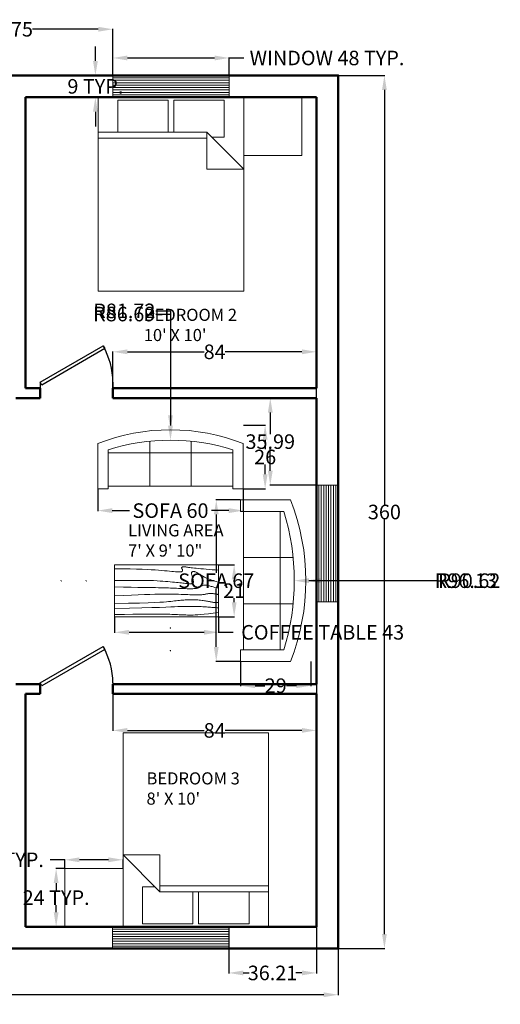
# Model space of a CAD drawing. Units: inches. Extents: x -8 to 445, y -363 to 43.
# Tile 3 of 3: x 246 to 445, y -363 to 43. Entities that reach past the tile are written whole.
import ezdxf

# ---------------------------------------------------------------- set-up
doc = ezdxf.new("R2010")
doc.units = ezdxf.units.IN
doc.header["$MEASUREMENT"] = 0
for name, color, linetype, lineweight in [('A-ANNO-DIMS', 2, 'Continuous', 18), ('A-AREA-IDEN', 7, 'Continuous', 18), ('A-FURN', 8, 'Continuous', 18), ('A-WALL', 7, 'Continuous', 50), ('DOORS', 43, 'Continuous', 25), ('WINDOWS', 140, 'Continuous', 18)]:
    doc.layers.add(name, color=color, linetype=linetype, lineweight=lineweight)
doc.styles.get("Standard").update_dxf_attribs({"font": 'arial.ttf'})
doc.dimstyles.get("Standard").update_dxf_attribs({"dimtxt": 6, "dimasz": 6, "dimexe": 0.18, "dimexo": 0.0625, "dimgap": 0.09, "dimtad": 0, "dimtih": 1, "dimtoh": 1, "dimdec": 0, "dimzin": 0, "dimdsep": 46, "dimlunit": 4, "dimtxsty": 'Standard', "dimcen": 0.09, "dimadec": 0, "dimazin": 0, "dimtfac": 1, "dimtdec": 0, "dimtofl": 0, "dimtmove": 0, "dimatfit": 3, "dimfxl": 1, "dimtolj": 1, "dimtzin": 0, "dimarcsym": 0})

# ---------------------------------------------------------------- blocks, each defined once
blk = doc.blocks.new('*U2')
for p, q in [((0, 0), (0, -6)), ((40, 0), (40, -6))]:
    blk.add_line(p, q)
blk.add_lwpolyline([(0, 0), (34.64, 20), (35.52, 18.48), (0.87, -1.52)], close=True)
blk.add_arc((0, 0), 40, 0, 30)
blk = doc.blocks.new('Sofa - Roundback 7 ft.')
for p, q in [((-12.00002, -32.4421), (-12.00003, -6.5971)), ((11.99997, -32.4421), (11.99998, -6.5971)), ((-36.000027, -34), (-36.000027, -11.4696)), ((-35.999844, -13.3819), (35.9998, -13.3819)), ((35.99998, -34), (35.99998, -11.4696)), ((-36.000027, -32.4421), (35.99998, -32.4421))]:
    blk.add_line(p, q)
for points in [[(-36.000027, -34), (-42.000027, -34), (-42.000027, -8)], [(41.99998, -8), (41.99998, -34), (35.99998, -34)]]:
    blk.add_lwpolyline(points)
for centre, radius, start, end in [((0, -114.25), 114.25, 68.43141, 111.5686), ((-0.00001, -127.1968), 121.1968, 72.72033, 107.2797)]:
    blk.add_arc(centre, radius, start, end)
blk = doc.blocks.new('Table - Rectangular Woodgrain 60 x 30 in.')
for p, q in [((0, 0), (0, -30)), ((60, 0), (0, 0)), ((60, -30), (60, 0)), ((0, -30), (60, -30))]:
    blk.add_line(p, q)
for points in [[(0, -2.4), (4.8155, -2.418), (9.0302, -2.4688), (12.709, -2.5477), (15.9167, -2.65), (18.7181, -2.7711), (21.1781, -2.9063), (23.3616, -3.0508), (25.3333, -3.2), (27.1477, -3.3495), (28.8172, -3.4958), (30.3437, -3.636), (31.7291, -3.7667), (32.9756, -3.8849), (34.0849, -3.9875), (35.059, -4.0714), (35.9, -4.1334), (36.6114, -4.1711), (37.2041, -4.1854), (37.6906, -4.1779), (38.0833, -4.15), (38.3948, -4.1034), (38.6375, -4.0396), (38.8239, -3.9602), (38.9666, -3.8667), (39.0764, -3.7608), (39.1573, -3.6448), (39.2116, -3.521), (39.2416, -3.3917), (39.2498, -3.2593), (39.2385, -3.1261), (39.21, -2.9944), (39.1666, -2.8667), (39.111, -2.7447), (39.0468, -2.6281), (38.978, -2.5163), (38.9083, -2.4083), (38.8418, -2.3035), (38.7823, -2.201), (38.7337, -2.1001), (38.7, -2), (38.6844, -1.9003), (38.6875, -1.8021), (38.7094, -1.707), (38.75, -1.6167), (38.8094, -1.5326), (38.8875, -1.4563), (38.9844, -1.3893), (39.1, -1.3333), (39.2351, -1.2896), (39.3937, -1.2583), (39.5804, -1.2396), (39.8, -1.2333), (40.057, -1.2396), (40.3562, -1.2583), (40.7023, -1.2896), (41.1, -1.3333), (41.5547, -1.3895), (42.0755, -1.4573), (42.6721, -1.5361), (43.3542, -1.625), (44.1316, -1.7233), (45.014, -1.8302), (46.0114, -1.9449), (47.1333, -2.0667), (48.3862, -2.1947), (49.7625, -2.3281), (51.2513, -2.4663), (52.8416, -2.6083), (54.5226, -2.7535), (56.2833, -2.9011), (58.1127, -3.0501), (60, -3.2)], [(0, -9.2), (6.5759, -9.0858), (11.9385, -9.0365), (16.2527, -9.0418), (19.6833, -9.0917), (22.3952, -9.1759), (24.5531, -9.2844), (26.322, -9.4069), (27.8666, -9.5333), (29.3241, -9.6553), (30.7203, -9.7719), (32.0532, -9.8837), (33.3208, -9.9917), (34.5213, -10.0965), (35.6526, -10.199), (36.7128, -10.2999), (37.7, -10.4), (38.6129, -10.4996), (39.4531, -10.5969), (40.223, -10.6895), (40.925, -10.775), (41.5613, -10.8512), (42.1344, -10.9156), (42.6465, -10.966), (43.1, -11), (43.4976, -11.0158), (43.8437, -11.0136), (44.143, -10.9942), (44.4, -10.9583), (44.6195, -10.9069), (44.8062, -10.8406), (44.9648, -10.7603), (45.1, -10.6667), (45.2155, -10.5598), (45.3114, -10.4365), (45.3871, -10.2929), (45.4416, -10.125), (45.4743, -9.929), (45.4844, -9.7011), (45.4709, -9.4371), (45.4333, -9.1333), (45.3716, -8.7883), (45.2896, -8.4104), (45.1919, -8.0107), (45.0833, -7.6), (44.9685, -7.1893), (44.8521, -6.7896), (44.7388, -6.4117), (44.6333, -6.0667), (44.54, -5.7628), (44.4614, -5.4979), (44.4001, -5.2675), (44.3583, -5.0667), (44.3384, -4.8909), (44.3427, -4.7354), (44.3736, -4.5956), (44.4333, -4.4667), (44.5236, -4.3453), (44.6427, -4.2333), (44.7884, -4.1339), (44.9583, -4.05), (45.1501, -3.9849), (45.3614, -3.9417), (45.59, -3.9234), (45.8333, -3.9333), (46.0915, -3.9749), (46.3734, -4.0531), (46.6906, -4.1736), (47.0542, -4.3417), (47.4756, -4.5629), (47.9661, -4.8427), (48.5372, -5.1866), (49.2, -5.6), (49.9676, -6.0844), (50.8594, -6.625), (51.8965, -7.2031), (53.1, -7.8), (54.491, -8.3969), (56.0906, -8.975), (57.9199, -9.5156), (60, -10)], [(0, -12.8), (5.1847, -12.9322), (9.6213, -13.0323), (13.3963, -13.1059), (16.5958, -13.1583), (19.3063, -13.1952), (21.614, -13.2219), (23.6054, -13.2439), (25.3666, -13.2667), (26.9728, -13.2947), (28.4531, -13.3281), (29.8256, -13.3663), (31.1083, -13.4083), (32.3191, -13.4535), (33.476, -13.501), (34.597, -13.5501), (35.7, -13.6), (36.7984, -13.6497), (37.8875, -13.6979), (38.9578, -13.743), (40, -13.7833), (41.0047, -13.8174), (41.9625, -13.8438), (42.864, -13.8607), (43.7, -13.8667), (44.4631, -13.8604), (45.1552, -13.8417), (45.7801, -13.8104), (46.3416, -13.7667), (46.8439, -13.7104), (47.2906, -13.6417), (47.6858, -13.5604), (48.0333, -13.4667), (48.3375, -13.3608), (48.6042, -13.2448), (48.8396, -13.121), (49.05, -12.9917), (49.2417, -12.8593), (49.4208, -12.7261), (49.5937, -12.5944), (49.7667, -12.4667), (49.9452, -12.3451), (50.1323, -12.2313), (50.3303, -12.1268), (50.5416, -12.0333), (50.7686, -11.9524), (51.0135, -11.8854), (51.2788, -11.8341), (51.5666, -11.8), (51.8785, -11.7843), (52.2116, -11.7865), (52.562, -11.8059), (52.926, -11.8417), (53.2998, -11.8931), (53.6795, -11.9594), (54.0614, -12.0397), (54.4416, -12.1333), (54.8223, -12.2401), (55.2293, -12.3625), (55.6942, -12.5037), (56.2489, -12.6667), (56.9251, -12.8547), (57.7545, -13.0708), (58.7689, -13.3182), (60, -13.6)], [(0, -18), (5.124, -17.7273), (9.6609, -17.5057), (13.6705, -17.3303), (17.2125, -17.1958), (20.3467, -17.0973), (23.1328, -17.0297), (25.6307, -16.9878), (27.9, -16.9667), (29.9928, -16.9617), (31.9302, -16.9703), (33.7254, -16.9907), (35.3917, -17.0208), (36.9423, -17.0588), (38.3906, -17.1026), (39.7499, -17.1503), (41.0333, -17.2), (42.2519, -17.2496), (43.4073, -17.2969), (44.4986, -17.3395), (45.525, -17.375), (46.4858, -17.4012), (47.3802, -17.4156), (48.2074, -17.416), (48.9667, -17.4), (49.6583, -17.3662), (50.2872, -17.3167), (50.8595, -17.2547), (51.3812, -17.1833), (51.8584, -17.1057), (52.2971, -17.025), (52.7034, -16.9443), (53.0833, -16.8667), (53.443, -16.7951), (53.789, -16.7313), (54.128, -16.6768), (54.4666, -16.6334), (54.8115, -16.6024), (55.1693, -16.5854), (55.5465, -16.5841), (55.95, -16.6), (56.3828, -16.6337), (56.8346, -16.6823), (57.2915, -16.7418), (57.7396, -16.8084), (58.165, -16.878), (58.5539, -16.9469), (58.8924, -17.0111), (59.1666, -17.0667), (59.3679, -17.1107), (59.5078, -17.1438), (59.6032, -17.1675), (59.6708, -17.1833), (59.7275, -17.193), (59.7901, -17.1979), (59.8753, -17.1998), (60, -17.2)], [(0, -22.4), (8.0098, -22.2501), (14.4094, -22.1011), (19.4168, -21.9535), (23.25, -21.8083), (26.1269, -21.6663), (28.2656, -21.5281), (29.884, -21.3947), (31.2, -21.2667), (32.3967, -21.1448), (33.5172, -21.0292), (34.5697, -20.9198), (35.5625, -20.8167), (36.5037, -20.7198), (37.4015, -20.6292), (38.2642, -20.5448), (39.1, -20.4667), (39.9164, -20.3951), (40.7187, -20.3313), (41.5117, -20.2768), (42.3, -20.2333), (43.0883, -20.2024), (43.8812, -20.1854), (44.6836, -20.1841), (45.5, -20.2), (46.3328, -20.234), (47.1747, -20.2844), (48.0163, -20.3488), (48.8479, -20.425), (49.66, -20.5106), (50.4429, -20.6031), (51.1872, -20.7004), (51.8833, -20.8), (52.5246, -20.8999), (53.1166, -20.9995), (53.6681, -21.0983), (54.1875, -21.1958), (54.6834, -21.2919), (55.1646, -21.3859), (55.6394, -21.4777), (56.1167, -21.5667), (56.6028, -21.6515), (57.0961, -21.7266), (57.5929, -21.7852), (58.0896, -21.8208), (58.5823, -21.8268), (59.0674, -21.7964), (59.5412, -21.723), (60, -21.6)], [(0, -25.2), (8.6355, -25.0504), (15.7026, -24.9031), (21.4049, -24.7606), (25.9458, -24.625), (29.529, -24.4988), (32.3578, -24.3844), (34.6359, -24.284), (36.5667, -24.2), (38.3213, -24.1341), (39.9417, -24.0854), (41.437, -24.0523), (42.8167, -24.0333), (44.0901, -24.0268), (45.2667, -24.0313), (46.3557, -24.0451), (47.3667, -24.0667), (48.309, -24.0947), (49.1928, -24.1287), (50.0284, -24.168), (50.826, -24.2125), (51.5959, -24.2617), (52.3483, -24.3151), (53.0935, -24.3725), (53.8417, -24.4334), (54.6009, -24.497), (55.3699, -24.561), (56.1454, -24.6226), (56.9239, -24.6792), (57.7021, -24.7279), (58.4764, -24.7662), (59.2435, -24.7911), (60, -24.8)], [(0, -28.8), (5.6867, -28.6681), (10.45, -28.5698), (14.407, -28.5012), (17.675, -28.4584), (20.3711, -28.4374), (22.6125, -28.4344), (24.5164, -28.4455), (26.2, -28.4667), (27.762, -28.4947), (29.2276, -28.5281), (30.6033, -28.5663), (31.8958, -28.6084), (33.1118, -28.6535), (34.2578, -28.7011), (35.3405, -28.7501), (36.3666, -28.8), (37.3443, -28.8497), (38.288, -28.8974), (39.2137, -28.9412), (40.1375, -28.9792), (41.0753, -29.0093), (42.0432, -29.0297), (43.0572, -29.0384), (44.1333, -29.0333), (45.2936, -29.0114), (46.5843, -28.9641), (48.0579, -28.8816), (49.7666, -28.7542), (51.7629, -28.5721), (54.0989, -28.3255), (56.8272, -28.0048), (60, -27.6)]]:
    blk.add_lwpolyline(points)
blk = doc.blocks.new('Bed - Queen')
for p, q in [((0, -80.00003), (0, 0)), ((0, 0), (59.99999, 0)), ((59.99999, 0), (59.99999, -80.00003)), ((7.99999, -1.2), (28.79998, -1.2)), ((7.99999, -14.4), (7.99999, -1.2)), ((28.79998, -1.2), (28.79998, -14.4)), ((31.19999, -1.2), (51.99999, -1.2)), ((31.19999, -14.4), (31.19999, -1.2)), ((51.99999, -1.2), (51.99999, -16.4)), ((0, -14.4), (44.8, -14.4)), ((59.99999, -29.6), (44.8, -14.4)), ((44.8, -14.4), (44.8, -29.6)), ((44.8, -16.8), (0, -16.8)), ((51.99999, -16.4), (46.79936, -16.4)), ((44.8, -29.6), (59.99999, -29.6)), ((59.99999, -80.00003), (0, -80.00003))]:
    blk.add_line(p, q)
blk = doc.blocks.new('WIN-48IN')
for p, q in [((0, 0), (0, 9)), ((0, 9), (48, 9)), ((48, 9), (48, 0)), ((0, 8), (48, 8)), ((0, 7), (48, 7)), ((0, 6), (48, 6)), ((0, 5), (48, 5)), ((0, 4), (48, 4)), ((0, 3), (48, 3)), ((0, 2), (48, 2)), ((48, 1), (0, 1)), ((48, 0), (0, 0))]:
    blk.add_line(p, q)
blk = doc.blocks.new('NIGHTSTAND-24IN')
blk.add_lwpolyline([(0, 24), (24, 24), (24, 0), (0, 0)], close=True)
blk = doc.blocks.new('*D15')
at = {"layer": 'A-ANNO-DIMS', "color": 0, "lineweight": -2, "transparency": 16777216}
for p, q in [((284.89, 19.97), (284.89, 27.29)), ((290.89, 27.11), (326.89, 27.11)), ((332.89, 19.97), (332.89, 27.29)), ((332.89, 27.11), (338.89, 27.11))]:
    blk.add_line(p, q, dxfattribs=at)
at = {"layer": 'A-ANNO-DIMS', "color": 0, "transparency": 16777216}
for points in [[(290.89, 28.11), (290.89, 26.11), (284.89, 27.11)], [(326.89, 28.11), (326.89, 26.11), (332.89, 27.11)]]:
    blk.add_solid(points, dxfattribs=at)
at = {"layer": 'Defpoints', "color": 0, "transparency": 16777216}
for p in [(332.89, 27.11), (284.89, 19.91), (332.89, 19.91)]:
    blk.add_point(p, dxfattribs=at)
at = {"layer": 'A-ANNO-DIMS', "color": 0, "transparency": 16777216, "insert": (373.26, 27.11), "char_height": 6, "attachment_point": 5}
blk.add_mtext('\\A1;WINDOW 48 TYP.', dxfattribs=at)
blk = doc.blocks.new('*D16')
at = {"layer": 'A-ANNO-DIMS', "color": 0, "lineweight": -2, "transparency": 16777216}
for p, q in [((277.69, 25.91), (277.69, 31.91)), ((284.82, 19.91), (277.51, 19.91)), ((284.82, 10.91), (277.51, 10.91)), ((277.69, 4.91), (277.69, -1.09))]:
    blk.add_line(p, q, dxfattribs=at)
at = {"layer": 'A-ANNO-DIMS', "color": 0, "transparency": 16777216}
for points in [[(276.69, 25.91), (278.69, 25.91), (277.69, 19.91)], [(276.69, 4.91), (278.69, 4.91), (277.69, 10.91)]]:
    blk.add_solid(points, dxfattribs=at)
at = {"layer": 'Defpoints', "color": 0, "transparency": 16777216}
for p in [(277.69, 19.91), (284.89, 19.91), (284.89, 10.91)]:
    blk.add_point(p, dxfattribs=at)
at = {"layer": 'A-ANNO-DIMS', "color": 0, "transparency": 16777216, "insert": (277.69, 15.41), "char_height": 6, "attachment_point": 5}
blk.add_mtext('\\A1;9 TYP.', dxfattribs=at)
blk = doc.blocks.new('*D19')
at = {"layer": 'A-ANNO-DIMS', "color": 0, "lineweight": -2, "transparency": 16777216}
for p, q in [((265.09, -303.49), (259.09, -303.49)), ((265.09, -307.03), (265.09, -303.31)), ((283.09, -303.49), (271.09, -303.49)), ((289.09, -307.03), (289.09, -303.31))]:
    blk.add_line(p, q, dxfattribs=at)
at = {"layer": 'A-ANNO-DIMS', "color": 0, "transparency": 16777216}
for points in [[(271.09, -302.49), (271.09, -304.49), (265.09, -303.49)], [(283.09, -302.49), (283.09, -304.49), (289.09, -303.49)]]:
    blk.add_solid(points, dxfattribs=at)
at = {"layer": 'Defpoints', "color": 0, "transparency": 16777216}
for p in [(265.09, -303.49), (265.09, -307.09), (289.09, -307.09)]:
    blk.add_point(p, dxfattribs=at)
at = {"layer": 'A-ANNO-DIMS', "color": 0, "transparency": 16777216, "insert": (216.13, -303.49), "char_height": 6, "attachment_point": 5}
blk.add_mtext('\\A1;NIGHTSTAND 24 TYP.', dxfattribs=at)
blk = doc.blocks.new('*D20')
at = {"layer": 'A-ANNO-DIMS', "color": 0, "lineweight": -2, "transparency": 16777216}
for p, q in [((265.02, -307.09), (261.31, -307.09)), ((261.49, -313.09), (261.49, -315.99)), ((261.49, -325.09), (261.49, -322.2)), ((265.02, -331.09), (261.31, -331.09))]:
    blk.add_line(p, q, dxfattribs=at)
at = {"layer": 'A-ANNO-DIMS', "color": 0, "transparency": 16777216}
for points in [[(260.49, -313.09), (262.49, -313.09), (261.49, -307.09)], [(260.49, -325.09), (262.49, -325.09), (261.49, -331.09)]]:
    blk.add_solid(points, dxfattribs=at)
at = {"layer": 'Defpoints', "color": 0, "transparency": 16777216}
for p in [(265.09, -307.09), (261.49, -331.09), (265.09, -331.09)]:
    blk.add_point(p, dxfattribs=at)
at = {"layer": 'A-ANNO-DIMS', "color": 0, "transparency": 16777216, "insert": (261.49, -319.09), "char_height": 6, "attachment_point": 5}
blk.add_mtext('\\A1;24 TYP.', dxfattribs=at)
blk = doc.blocks.new('*D21')
at = {"layer": 'A-ANNO-DIMS', "color": 0, "lineweight": -2, "transparency": 16777216}
for p, q in [((337.49, -155.1), (327.38, -155.1)), ((327.56, -161.1), (327.56, -185.21)), ((327.56, -215.72), (327.56, -191.6)), ((337.49, -221.72), (327.38, -221.72))]:
    blk.add_line(p, q, dxfattribs=at)
at = {"layer": 'A-ANNO-DIMS', "color": 0, "transparency": 16777216}
for points in [[(326.56, -161.1), (328.56, -161.1), (327.56, -155.1)], [(326.56, -215.72), (328.56, -215.72), (327.56, -221.72)]]:
    blk.add_solid(points, dxfattribs=at)
at = {"layer": 'Defpoints', "color": 0, "transparency": 16777216}
for p in [(337.55, -155.1), (327.56, -221.72), (337.55, -221.72)]:
    blk.add_point(p, dxfattribs=at)
at = {"layer": 'A-ANNO-DIMS', "color": 0, "transparency": 16777216, "insert": (327.56, -188.41), "char_height": 6, "attachment_point": 5}
blk.add_mtext('\\A1;SOFA 67', dxfattribs=at)
blk = doc.blocks.new('*D22')
at = {"layer": 'A-ANNO-DIMS', "color": 0, "lineweight": -2, "transparency": 16777216}
for p, q in [((337.55, -221.78), (337.55, -231.89)), ((366.63, -221.78), (366.63, -231.89)), ((343.55, -231.71), (347.65, -231.71)), ((360.63, -231.71), (356.54, -231.71))]:
    blk.add_line(p, q, dxfattribs=at)
at = {"layer": 'A-ANNO-DIMS', "color": 0, "transparency": 16777216}
for points in [[(343.55, -230.71), (343.55, -232.71), (337.55, -231.71)], [(360.63, -230.71), (360.63, -232.71), (366.63, -231.71)]]:
    blk.add_solid(points, dxfattribs=at)
at = {"layer": 'Defpoints', "color": 0, "transparency": 16777216}
for p in [(337.55, -221.72), (366.63, -221.72), (366.63, -231.71)]:
    blk.add_point(p, dxfattribs=at)
at = {"layer": 'A-ANNO-DIMS', "color": 0, "transparency": 16777216, "insert": (352.09, -231.71), "char_height": 6, "attachment_point": 5}
blk.add_mtext('\\A1;29', dxfattribs=at)
blk = doc.blocks.new('*D23')
at = {"layer": 'A-ANNO-DIMS', "color": 0, "lineweight": -2, "transparency": 16777216}
for p, q in [((278.63, -150.57), (278.63, -159.7)), ((338.71, -150.57), (338.71, -159.7)), ((284.63, -159.52), (291.74, -159.52)), ((332.71, -159.52), (325.61, -159.52))]:
    blk.add_line(p, q, dxfattribs=at)
at = {"layer": 'A-ANNO-DIMS', "color": 0, "transparency": 16777216}
for points in [[(284.63, -158.52), (284.63, -160.52), (278.63, -159.52)], [(332.71, -158.52), (332.71, -160.52), (338.71, -159.52)]]:
    blk.add_solid(points, dxfattribs=at)
at = {"layer": 'Defpoints', "color": 0, "transparency": 16777216}
for p in [(278.63, -150.51), (338.71, -150.51), (338.71, -159.52)]:
    blk.add_point(p, dxfattribs=at)
at = {"layer": 'A-ANNO-DIMS', "color": 0, "transparency": 16777216, "insert": (308.67, -159.52), "char_height": 6, "attachment_point": 5}
blk.add_mtext('\\A1;SOFA 60', dxfattribs=at)
blk = doc.blocks.new('*D24')
at = {"layer": 'A-ANNO-DIMS', "color": 0, "lineweight": -2, "transparency": 16777216}
for p, q in [((338.78, -124.28), (347.91, -124.28)), ((347.73, -130.28), (347.73, -134.24)), ((347.73, -144.51), (347.73, -140.55)), ((338.78, -150.51), (347.91, -150.51))]:
    blk.add_line(p, q, dxfattribs=at)
at = {"layer": 'A-ANNO-DIMS', "color": 0, "transparency": 16777216}
for points in [[(346.73, -130.28), (348.73, -130.28), (347.73, -124.28)], [(346.73, -144.51), (348.73, -144.51), (347.73, -150.51)]]:
    blk.add_solid(points, dxfattribs=at)
at = {"layer": 'Defpoints', "color": 0, "transparency": 16777216}
for p in [(338.71, -124.28), (347.73, -124.28), (338.71, -150.51)]:
    blk.add_point(p, dxfattribs=at)
at = {"layer": 'A-ANNO-DIMS', "color": 0, "transparency": 16777216, "insert": (347.73, -137.4), "char_height": 6, "attachment_point": 5}
blk.add_mtext('\\A1;26', dxfattribs=at)
blk = doc.blocks.new('*D25')
at = {"layer": 'A-ANNO-DIMS', "color": 0, "lineweight": -2, "transparency": 16777216}
for p, q in [((285.61, -203.33), (285.61, -209.88)), ((328.51, -203.33), (328.51, -209.88)), ((291.61, -209.7), (322.51, -209.7)), ((328.51, -209.7), (334.51, -209.7))]:
    blk.add_line(p, q, dxfattribs=at)
at = {"layer": 'A-ANNO-DIMS', "color": 0, "transparency": 16777216}
for points in [[(291.61, -208.7), (291.61, -210.7), (285.61, -209.7)], [(322.51, -208.7), (322.51, -210.7), (328.51, -209.7)]]:
    blk.add_solid(points, dxfattribs=at)
at = {"layer": 'Defpoints', "color": 0, "transparency": 16777216}
for p in [(285.61, -203.27), (328.51, -203.27), (328.51, -209.7)]:
    blk.add_point(p, dxfattribs=at)
at = {"layer": 'A-ANNO-DIMS', "color": 0, "transparency": 16777216, "insert": (371.47, -209.7), "char_height": 6, "attachment_point": 5}
blk.add_mtext('\\A1;COFFEE TABLE 43', dxfattribs=at)
blk = doc.blocks.new('*D26')
at = {"layer": 'A-ANNO-DIMS', "color": 0, "lineweight": -2, "transparency": 16777216}
for p, q in [((328.58, -181.81), (335.13, -181.81)), ((334.95, -187.81), (334.95, -189.44)), ((334.95, -197.27), (334.95, -195.64)), ((328.58, -203.27), (335.13, -203.27))]:
    blk.add_line(p, q, dxfattribs=at)
at = {"layer": 'A-ANNO-DIMS', "color": 0, "transparency": 16777216}
for points in [[(333.95, -187.81), (335.95, -187.81), (334.95, -181.81)], [(333.95, -197.27), (335.95, -197.27), (334.95, -203.27)]]:
    blk.add_solid(points, dxfattribs=at)
at = {"layer": 'Defpoints', "color": 0, "transparency": 16777216}
for p in [(328.51, -181.81), (334.95, -181.81), (328.51, -203.27)]:
    blk.add_point(p, dxfattribs=at)
at = {"layer": 'A-ANNO-DIMS', "color": 0, "transparency": 16777216, "insert": (334.95, -192.54), "char_height": 6, "attachment_point": 5}
blk.add_mtext('\\A1;21', dxfattribs=at)
blk = doc.blocks.new('*D33')
at = {"layer": 'A-ANNO-DIMS', "color": 0, "lineweight": -2, "transparency": 16777216}
for p, q in [((17.89, -340.15), (17.89, -359.32)), ((377.89, -340.15), (377.89, -359.32)), ((23.89, -359.14), (191.18, -359.14)), ((371.89, -359.14), (204.59, -359.14))]:
    blk.add_line(p, q, dxfattribs=at)
at = {"layer": 'A-ANNO-DIMS', "color": 0, "transparency": 16777216}
for points in [[(23.89, -358.14), (23.89, -360.14), (17.89, -359.14)], [(371.89, -358.14), (371.89, -360.14), (377.89, -359.14)]]:
    blk.add_solid(points, dxfattribs=at)
at = {"layer": 'Defpoints', "color": 0, "transparency": 16777216}
for p in [(17.89, -340.09), (377.89, -340.09), (377.89, -359.14)]:
    blk.add_point(p, dxfattribs=at)
at = {"layer": 'A-ANNO-DIMS', "color": 0, "transparency": 16777216, "insert": (197.89, -359.14), "char_height": 6, "attachment_point": 5}
blk.add_mtext('\\A1;360', dxfattribs=at)
blk = doc.blocks.new('*D34')
at = {"layer": 'A-ANNO-DIMS', "color": 0, "lineweight": -2, "transparency": 16777216}
for p, q in [((377.95, 19.91), (397.12, 19.91)), ((396.94, 13.91), (396.94, -156.94)), ((396.94, -334.09), (396.94, -163.25)), ((377.95, -340.09), (397.12, -340.09))]:
    blk.add_line(p, q, dxfattribs=at)
at = {"layer": 'A-ANNO-DIMS', "color": 0, "transparency": 16777216}
for points in [[(395.94, 13.91), (397.94, 13.91), (396.94, 19.91)], [(395.94, -334.09), (397.94, -334.09), (396.94, -340.09)]]:
    blk.add_solid(points, dxfattribs=at)
at = {"layer": 'Defpoints', "color": 0, "transparency": 16777216}
for p in [(377.89, 19.91), (396.94, 19.91), (377.89, -340.09)]:
    blk.add_point(p, dxfattribs=at)
at = {"layer": 'A-ANNO-DIMS', "color": 0, "transparency": 16777216, "insert": (396.94, -160.09), "char_height": 6, "attachment_point": 5}
blk.add_mtext('\\A1;360', dxfattribs=at)
blk = doc.blocks.new('*D38')
at = {"layer": 'A-ANNO-DIMS', "color": 0, "lineweight": -2, "transparency": 16777216}
for p, q in [((209.89, 19.97), (209.89, 39.14)), ((215.89, 38.96), (243, 38.96)), ((278.89, 38.96), (251.77, 38.96)), ((284.89, 19.97), (284.89, 39.14))]:
    blk.add_line(p, q, dxfattribs=at)
at = {"layer": 'A-ANNO-DIMS', "color": 0, "transparency": 16777216}
for points in [[(215.89, 39.96), (215.89, 37.96), (209.89, 38.96)], [(278.89, 39.96), (278.89, 37.96), (284.89, 38.96)]]:
    blk.add_solid(points, dxfattribs=at)
at = {"layer": 'Defpoints', "color": 0, "transparency": 16777216}
for p in [(284.89, 38.96), (209.89, 19.91), (284.89, 19.91)]:
    blk.add_point(p, dxfattribs=at)
at = {"layer": 'A-ANNO-DIMS', "color": 0, "transparency": 16777216, "insert": (247.39, 38.96), "char_height": 6, "attachment_point": 5}
blk.add_mtext('\\A1;75', dxfattribs=at)
blk = doc.blocks.new('*D45')
at = {"layer": 'A-ANNO-DIMS', "color": 0, "lineweight": -2, "transparency": 16777216}
for p, q in [((368.82, -113.09), (349.66, -113.09)), ((349.84, -119.09), (349.84, -127.93)), ((349.84, -143.08), (349.84, -134.24)), ((368.82, -149.08), (349.66, -149.08))]:
    blk.add_line(p, q, dxfattribs=at)
at = {"layer": 'A-ANNO-DIMS', "color": 0, "transparency": 16777216}
for points in [[(348.84, -119.09), (350.84, -119.09), (349.84, -113.09)], [(348.84, -143.08), (350.84, -143.08), (349.84, -149.08)]]:
    blk.add_solid(points, dxfattribs=at)
at = {"layer": 'Defpoints', "color": 0, "transparency": 16777216}
for p in [(349.84, -113.09), (368.89, -113.09), (368.89, -149.08)]:
    blk.add_point(p, dxfattribs=at)
at = {"layer": 'A-ANNO-DIMS', "color": 0, "transparency": 16777216, "insert": (349.84, -131.08), "char_height": 6, "attachment_point": 5}
blk.add_mtext('\\A1;35.99', dxfattribs=at)
blk = doc.blocks.new('*D55')
at = {"layer": 'A-ANNO-DIMS', "color": 0, "lineweight": -2, "transparency": 16777216}
for p, q in [((284.89, -113.03), (284.89, -93.86)), ((290.89, -94.04), (322.51, -94.04)), ((362.89, -94.04), (331.27, -94.04)), ((368.89, -113.03), (368.89, -93.86))]:
    blk.add_line(p, q, dxfattribs=at)
at = {"layer": 'A-ANNO-DIMS', "color": 0, "transparency": 16777216}
for points in [[(290.89, -93.04), (290.89, -95.04), (284.89, -94.04)], [(362.89, -93.04), (362.89, -95.04), (368.89, -94.04)]]:
    blk.add_solid(points, dxfattribs=at)
at = {"layer": 'Defpoints', "color": 0, "transparency": 16777216}
for p in [(368.89, -94.04), (284.89, -113.09), (368.89, -113.09)]:
    blk.add_point(p, dxfattribs=at)
at = {"layer": 'A-ANNO-DIMS', "color": 0, "transparency": 16777216, "insert": (326.89, -94.04), "char_height": 6, "attachment_point": 5}
blk.add_mtext('\\A1;84', dxfattribs=at)
blk = doc.blocks.new('*D56')
at = {"layer": 'A-ANNO-DIMS', "color": 0, "lineweight": -2, "transparency": 16777216}
for p, q in [((284.89, -231.15), (284.89, -250.32)), ((368.89, -231.15), (368.89, -250.32)), ((290.89, -250.14), (322.51, -250.14)), ((362.89, -250.14), (331.27, -250.14))]:
    blk.add_line(p, q, dxfattribs=at)
at = {"layer": 'A-ANNO-DIMS', "color": 0, "transparency": 16777216}
for points in [[(290.89, -249.14), (290.89, -251.14), (284.89, -250.14)], [(362.89, -249.14), (362.89, -251.14), (368.89, -250.14)]]:
    blk.add_solid(points, dxfattribs=at)
at = {"layer": 'Defpoints', "color": 0, "transparency": 16777216}
for p in [(284.89, -231.09), (368.89, -231.09), (284.89, -250.14)]:
    blk.add_point(p, dxfattribs=at)
at = {"layer": 'A-ANNO-DIMS', "color": 0, "transparency": 16777216, "insert": (326.89, -250.14), "char_height": 6, "attachment_point": 5}
blk.add_mtext('\\A1;84', dxfattribs=at)
blk = doc.blocks.new('*D59')
at = {"layer": 'A-ANNO-DIMS', "color": 0, "lineweight": -2, "transparency": 16777216}
for p, q in [((332.68, -331.15), (332.68, -350.32)), ((368.89, -331.15), (368.89, -350.32)), ((338.68, -350.14), (341.15, -350.14)), ((362.89, -350.14), (360.42, -350.14))]:
    blk.add_line(p, q, dxfattribs=at)
at = {"layer": 'A-ANNO-DIMS', "color": 0, "transparency": 16777216}
for points in [[(338.68, -349.14), (338.68, -351.14), (332.68, -350.14)], [(362.89, -349.14), (362.89, -351.14), (368.89, -350.14)]]:
    blk.add_solid(points, dxfattribs=at)
at = {"layer": 'Defpoints', "color": 0, "transparency": 16777216}
for p in [(332.68, -331.09), (368.89, -331.09), (332.68, -350.14)]:
    blk.add_point(p, dxfattribs=at)
at = {"layer": 'A-ANNO-DIMS', "color": 0, "transparency": 16777216, "insert": (350.78, -350.14), "char_height": 6, "attachment_point": 5}
blk.add_mtext('\\A1;36.21', dxfattribs=at)
blk = doc.blocks.new('*D62')
at = {"layer": 'A-ANNO-DIMS', "color": 0, "lineweight": -2, "transparency": 16777216}
for p, q in [((263.54, -188.41), (263.72, -188.41)), ((263.63, -188.5), (263.63, -188.32)), ((417.44, -188.41), (365.76, -188.41))]:
    blk.add_line(p, q, dxfattribs=at)
at = {"layer": 'A-ANNO-DIMS', "color": 0, "transparency": 16777216}
blk.add_solid([(365.76, -187.41), (365.76, -189.41), (359.76, -188.41)], dxfattribs=at)
at = {"layer": 'Defpoints', "color": 0, "transparency": 16777216}
for p in [(263.63, -188.41), (359.76, -188.41)]:
    blk.add_point(p, dxfattribs=at)
at = {"layer": 'A-ANNO-DIMS', "color": 0, "transparency": 16777216, "insert": (430.52, -188.41), "char_height": 6, "attachment_point": 5}
blk.add_mtext('\\A1;R96.13', dxfattribs=at)
blk = doc.blocks.new('*D63')
at = {"layer": 'A-ANNO-DIMS', "color": 0, "lineweight": -2, "transparency": 16777216}
for p, q in [((273.81, -188.41), (273.99, -188.41)), ((273.9, -188.5), (273.9, -188.32)), ((418.89, -188.41), (370.52, -188.41))]:
    blk.add_line(p, q, dxfattribs=at)
at = {"layer": 'A-ANNO-DIMS', "color": 0, "transparency": 16777216}
blk.add_solid([(370.52, -187.41), (370.52, -189.41), (364.52, -188.41)], dxfattribs=at)
at = {"layer": 'Defpoints', "color": 0, "transparency": 16777216}
for p in [(273.9, -188.41), (364.52, -188.41)]:
    blk.add_point(p, dxfattribs=at)
at = {"layer": 'A-ANNO-DIMS', "color": 0, "transparency": 16777216, "insert": (431.94, -188.41), "char_height": 6, "attachment_point": 5}
blk.add_mtext('\\A1;R90.62', dxfattribs=at)
blk = doc.blocks.new('*D64')
at = {"layer": 'A-ANNO-DIMS', "color": 0, "lineweight": -2, "transparency": 16777216}
for p, q in [((302.67, -78.47), (308.67, -78.47)), ((308.67, -78.47), (308.67, -124.48)), ((308.58, -217.17), (308.76, -217.17)), ((308.67, -217.26), (308.67, -217.08))]:
    blk.add_line(p, q, dxfattribs=at)
at = {"layer": 'A-ANNO-DIMS', "color": 0, "transparency": 16777216}
blk.add_solid([(309.67, -124.48), (307.67, -124.48), (308.67, -130.48)], dxfattribs=at)
at = {"layer": 'Defpoints', "color": 0, "transparency": 16777216}
for p in [(308.67, -130.48), (308.67, -217.17)]:
    blk.add_point(p, dxfattribs=at)
at = {"layer": 'A-ANNO-DIMS', "color": 0, "transparency": 16777216, "insert": (289.58, -78.47), "char_height": 6, "attachment_point": 5}
blk.add_mtext('\\A1;R86.69', dxfattribs=at)
blk = doc.blocks.new('*D65')
at = {"layer": 'A-ANNO-DIMS', "color": 0, "lineweight": -2, "transparency": 16777216}
for p, q in [((302.67, -77.16), (308.67, -77.16)), ((308.67, -77.16), (308.67, -120.19)), ((308.58, -207.91), (308.76, -207.91)), ((308.67, -208), (308.67, -207.82))]:
    blk.add_line(p, q, dxfattribs=at)
at = {"layer": 'A-ANNO-DIMS', "color": 0, "transparency": 16777216}
blk.add_solid([(309.67, -120.19), (307.67, -120.19), (308.67, -126.19)], dxfattribs=at)
at = {"layer": 'Defpoints', "color": 0, "transparency": 16777216}
for p in [(308.67, -126.19), (308.67, -207.91)]:
    blk.add_point(p, dxfattribs=at)
at = {"layer": 'A-ANNO-DIMS', "color": 0, "transparency": 16777216, "insert": (289.62, -77.16), "char_height": 6, "attachment_point": 5}
blk.add_mtext('\\A1;R81.72', dxfattribs=at)

msp = doc.modelspace()

# ---------------------------------------------------------------- linework, layer by layer
at = {"layer": 'A-WALL'}
for p, q in [((248.8872, 10.9093), (248.8872, -109.0907)), ((248.8872, 10.9093), (368.8872, 10.9093)), ((368.8872, 10.9093), (368.8872, -109.0907)), ((248.8872, -109.0907), (254.8872, -109.0907)), ((254.8872, -113.0907), (254.8872, -109.0907)), ((284.8872, -113.0907), (284.8872, -109.0907)), ((284.8872, -109.0907), (368.8872, -109.0907)), ((244.8872, -113.0907), (254.8872, -113.0907)), ((248.8872, -113.0907), (254.8872, -113.0907)), ((284.8872, -113.0907), (368.8872, -113.0907)), ((284.8872, -113.0907), (368.8872, -113.0907)), ((368.8872, -113.0907), (368.8872, -231.0907)), ((254.8872, -231.0907), (244.8872, -231.0907)), ((254.8872, -231.0907), (248.8872, -231.0907)), ((254.8872, -235.0907), (254.8872, -231.0907)), ((368.8872, -231.0907), (284.8872, -231.0907)), ((368.8872, -231.0907), (284.8872, -231.0907)), ((284.8872, -235.0907), (284.8872, -231.0907)), ((248.8872, -235.0907), (248.8872, -331.0907)), ((254.8872, -235.0907), (248.8872, -235.0907)), ((368.8872, -235.0907), (284.8872, -235.0907)), ((368.8872, -235.0907), (368.8872, -331.0907)), ((368.8872, -331.0907), (248.8872, -331.0907))]:
    msp.add_line(p, q, dxfattribs=at)
msp.add_lwpolyline([(182.8872, -340.0907), (17.8872, -340.0907), (17.8872, 19.9093), (377.8872, 19.9093), (377.8872, -340.0907), (212.8872, -340.0907)], dxfattribs=at)

# ---------------------------------------------------------------- block references
at = {"layer": 'A-FURN'}
for name, p in [('Bed - Queen', (278.8872, 10.9093)), ('NIGHTSTAND-24IN', (338.887, -13.091))]:
    msp.add_blockref(name, p, dxfattribs=at)
for name, p, xscale, yscale, zscale in [('Sofa - Roundback 7 ft.', (308.6745, -126.1915), 0.7152482089798694, 0.7152482089798694, 0.7152482089798694), ('Table - Rectangular Woodgrain 60 x 30 in.', (285.6082, -181.8144), 0.7150895001404479, 0.7150895001404479, 0.7150895001404479)]:
    msp.add_blockref(name, p, dxfattribs=dict(at, xscale=xscale, yscale=yscale, zscale=zscale))
at = {"layer": 'A-FURN', "xscale": 0.793140179634724, "yscale": 0.793140179634724, "zscale": 0.793140179634724, "rotation": 270}
msp.add_blockref('Sofa - Roundback 7 ft.', (364.5196, -188.4084), dxfattribs=at)
at = {"layer": 'A-FURN', "rotation": 180}
for name, p in [('Bed - Queen', (349.0866, -331.0907)), ('NIGHTSTAND-24IN', (289.0868, -307.0904))]:
    msp.add_blockref(name, p, dxfattribs=at)
at = {"layer": 'DOORS', "xscale": 0.75, "yscale": 0.75, "zscale": 0.75}
for p in [(254.8872, -106.5907), (254.8872, -230.5907)]:
    msp.add_blockref('*U2', p, dxfattribs=at)
at = {"layer": 'WINDOWS'}
for p in [(284.887, 10.909), (284.6783, -340.091)]:
    msp.add_blockref('WIN-48IN', p, dxfattribs=at)
at = {"layer": 'WINDOWS', "rotation": 270}
msp.add_blockref('WIN-48IN', (368.8869, -149.0777), dxfattribs=at)

# ---------------------------------------------------------------- texts
at = {"layer": 'A-AREA-IDEN', "char_height": 5, "attachment_point": 1}
for s, width, insert in [("BEDROOM 2\\P10' X 10'", 74.42934, (297.6352, -76.2956)), ('LIVING AREA\\P7\' X 9\' 10"', 66.667723, (291.1527, -165.1525)), ("BEDROOM 3 \\P8' X 10'", 86.000919, (298.7739, -267.4284))]:
    msp.add_mtext_dynamic_manual_height_columns(s, width=width, gutter_width=1, heights=[0], dxfattribs=dict(at, insert=insert))

# ---------------------------------------------------------------- dimensions: what is measured, and where the dimension line sits
at = {"layer": 'A-ANNO-DIMS'}
for base, p1, p2, picture, middle in [((284.8872, 38.9593), (209.8872, 19.9093), (284.8872, 19.9093), '*D38', (247.3872, 38.9593)), ((368.8872, -94.0407), (284.8872, -113.0907), (368.8872, -113.0907), '*D55', (326.8872, -94.0407)), ((366.6346, -231.7139), (337.5528, -221.7203), (366.6346, -221.7203), '*D22', (352.0937, -231.7139)), ((377.8872, -359.1407), (17.8872, -340.0907), (377.8872, -340.0907), '*D33', (197.8872, -359.1407))]:
    dim = msp.add_linear_dim(base=base, p1=p1, p2=p2, dimstyle='Standard', override={"dimdec": 0, "dimlfac": 1, "dimrnd": 0, "dimzin": 0, "dimdsep": 46, "dimlunit": 2}, dxfattribs=at)
    dim.commit()
    dim.dimension.update_dxf_attribs({"geometry": picture, "text_midpoint": middle})
for base, p1, p2, text, picture, middle in [((332.8872, 27.1093), (284.8872, 19.9093), (332.8872, 19.9093), 'WINDOW <> TYP.', '*D15', (373.2562, 27.1093)), ((338.7149, -159.5221), (278.634, -150.5099), (338.7149, -150.5099), 'SOFA <>', '*D23', (308.6745, -159.5221)), ((328.5135, -209.7029), (285.6082, -203.2671), (328.5135, -203.2671), 'COFFEE TABLE <>', '*D25', (371.4692, -209.7029))]:
    dim = msp.add_linear_dim(base=base, p1=p1, p2=p2, text=text, dimstyle='Standard', override={"dimdec": 0, "dimlfac": 1, "dimrnd": 0, "dimzin": 0, "dimdsep": 46, "dimlunit": 2}, dxfattribs=at)
    dim.commit()
    dim.dimension.update_dxf_attribs({"geometry": picture, "text_midpoint": middle})
for base, p1, p2, angle, text, picture, middle in [((277.6872, 19.9093), (284.8872, 10.9093), (284.8872, 19.9093), 90, '<> TYP.', '*D16', (277.6872, 15.4093)), ((327.5593, -221.7203), (337.5528, -155.0965), (337.5528, -221.7203), 270, 'SOFA <>', '*D21', (327.5593, -188.4084)), ((265.0866, -303.4907), (289.0866, -307.0907), (265.0866, -307.0907), 180, 'NIGHTSTAND <> TYP.', '*D19', (216.133, -303.4907)), ((261.4866, -331.0907), (265.0866, -307.0907), (265.0866, -331.0907), 270, '<> TYP.', '*D20', (261.4866, -319.0907))]:
    dim = msp.add_linear_dim(base=base, p1=p1, p2=p2, angle=angle, text=text, dimstyle='Standard', override={"dimdec": 0, "dimlfac": 1, "dimrnd": 0, "dimzin": 0, "dimdsep": 46, "dimlunit": 2}, dxfattribs=at)
    dim.commit()
    dim.dimension.update_dxf_attribs({"geometry": picture, "text_midpoint": middle})
for base, p1, p2, angle, override, picture, middle in [((396.9372, 19.9093), (377.8872, -340.0907), (377.8872, 19.9093), 90, {"dimdec": 0, "dimlfac": 1, "dimrnd": 0, "dimzin": 0, "dimdsep": 46, "dimlunit": 2}, '*D34', (396.9372, -160.0907)), ((349.8372, -113.0907), (368.8872, -149.078), (368.8872, -113.0907), 90, {"dimdec": 2, "dimlfac": 1, "dimrnd": 0, "dimzin": 0, "dimdsep": 46, "dimlunit": 2}, '*D45', (349.8372, -131.0843)), ((347.727, -124.2842), (338.7149, -150.5099), (338.7149, -124.2842), 90, {"dimdec": 0, "dimlfac": 1, "dimrnd": 0, "dimzin": 0, "dimdsep": 46, "dimlunit": 2}, '*D24', (347.727, -137.3971)), ((334.9494, -181.8144), (328.5135, -203.2671), (328.5135, -181.8144), 90, {"dimdec": 0, "dimlfac": 1, "dimrnd": 0, "dimzin": 0, "dimdsep": 46, "dimlunit": 2}, '*D26', (334.9494, -192.5407)), ((284.8872, -250.1407), (368.8872, -231.0907), (284.8872, -231.0907), 180, {"dimdec": 0, "dimlfac": 1, "dimrnd": 0, "dimzin": 0, "dimdsep": 46, "dimlunit": 2}, '*D56', (326.8872, -250.1407)), ((332.6785, -350.1407), (368.8872, -331.0907), (332.6785, -331.0907), 180, {"dimdec": 2, "dimlfac": 1, "dimrnd": 0, "dimzin": 0, "dimdsep": 46, "dimlunit": 2}, '*D59', (350.7829, -350.1407))]:
    dim = msp.add_linear_dim(base=base, p1=p1, p2=p2, angle=angle, dimstyle='Standard', override=override, dxfattribs=at)
    dim.commit()
    dim.dimension.update_dxf_attribs({"geometry": picture, "text_midpoint": middle})
for center, mpoint, picture, middle in [((308.6745, -217.1688), (308.674, -130.483), '*D64', (289.583, -78.4715)), ((308.6745, -207.9086), (308.674, -126.1915), '*D65', (289.6199, -77.1612)), ((263.6347, -188.4084), (359.7608, -188.408), '*D62', (417.4364, -188.4078)), ((273.9033, -188.4084), (364.5196, -188.408), '*D63', (418.8894, -188.4077))]:
    dim = msp.add_radius_dim(center=center, mpoint=mpoint, dimstyle='Standard', override={"dimdec": 2, "dimlfac": 1, "dimrnd": 0, "dimzin": 0, "dimdsep": 46, "dimlunit": 2}, dxfattribs=at)
    dim.commit()
    dim.dimension.update_dxf_attribs({"geometry": picture, "text_midpoint": middle, "dimtype": 164})

doc.saveas('drawing.dxf')
